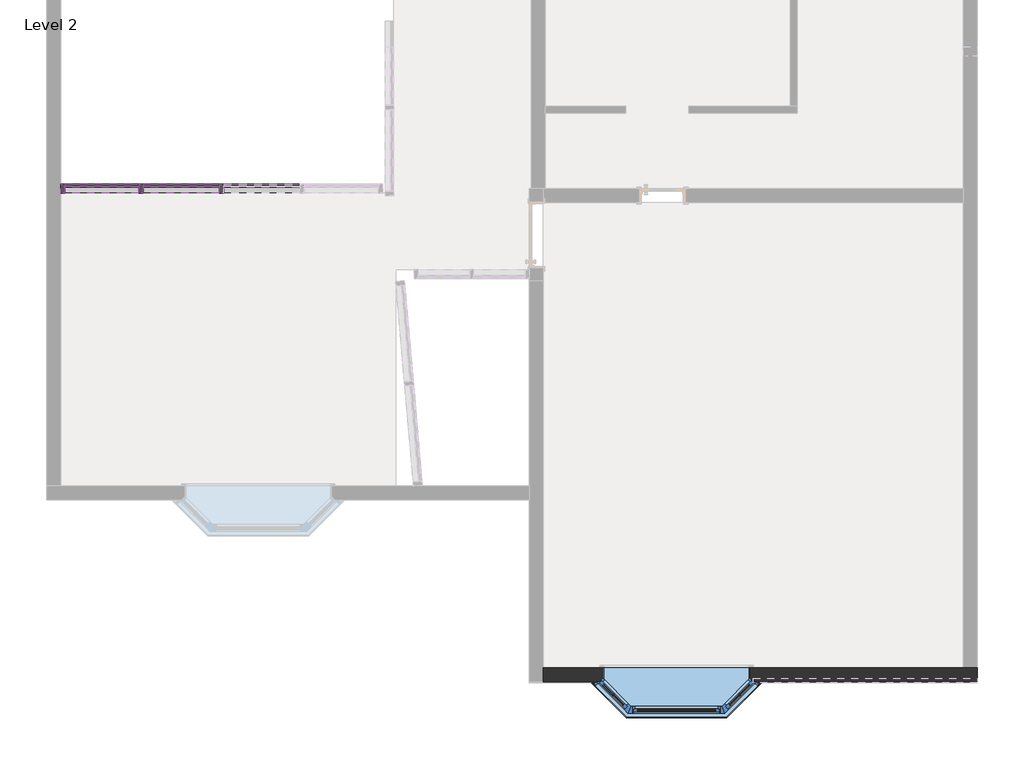
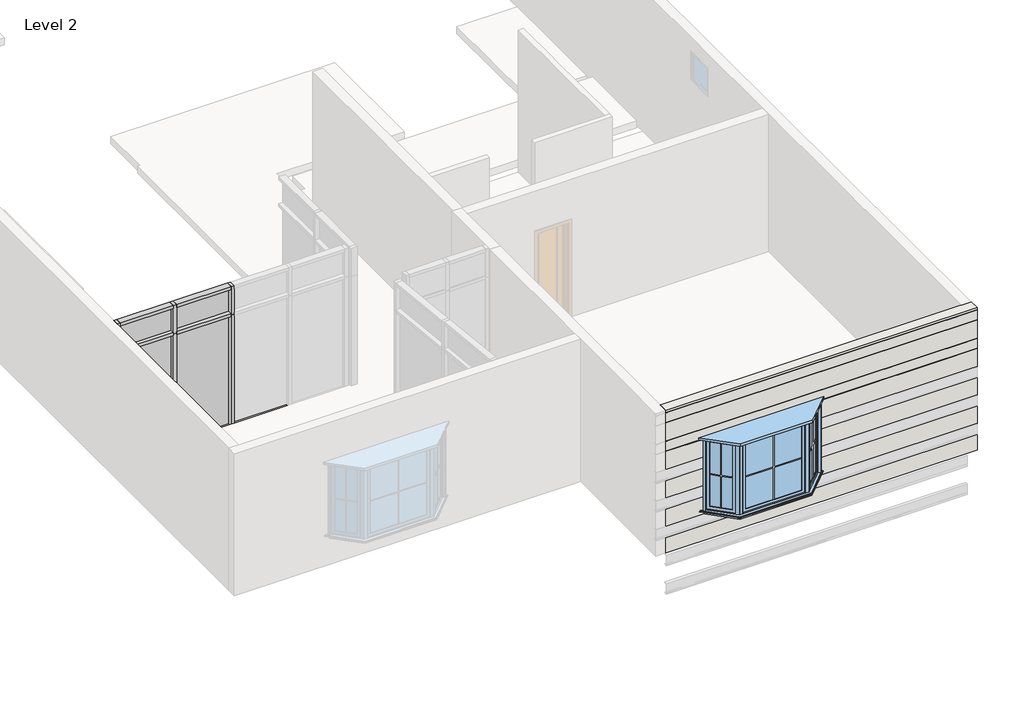
# One storey, part 1 of 5: 13 members, 4 plates, 1 wall, 1 window.
"""IFC4 building model written with IfcOpenShell, lengths in millimetres."""

from ifc_helpers import new_model, si_unit, frame, origin, place, context, project, spatial, polyline, circle_curve, ellipse_curve, transform, mapped, element, save
from ifc_brep_helpers import plane_surface, cylinder_surface, revolved_surface, advanced_brep
from components import member_47bfaf8a, member_ee409385, member_0d004d8a, member_f5e9651f, member_be44f791, member_766f1680, member_f0fea5a5, member_6e77e263, system_panel_glazed_2e981f09, system_panel_glazed_87980334, system_panel_glazed_ed20128f, system_panel_glazed_d57d3c71, window_9f89e8e4

model = new_model("IFC4")

# Units and contexts
model_context = context("Model", 3, world=origin())
ifc_project = project(units=[si_unit("LENGTHUNIT", "METRE", prefix="MILLI")], contexts=[model_context])

# Site, building, storey
site = spatial("IfcSite", under=ifc_project)
building = spatial("IfcBuilding", under=site)
storey = spatial("IfcBuildingStorey", under=building, Name="Level 2", Elevation=3048.0)

# Members
placement = place(None, origin())
member_shape = member_47bfaf8a(model_context)
element("IfcMember", 1, ObjectType="Rectangular Mullion : 2.5\" x 5\" rectangular", at=placement, inside=storey, context=model_context, shape_type="MappedRepresentation", body=[
    mapped(member_shape, transform((-50556.1380314, -2838.2913973, 6096.0), x_axis=(-1.0, 0.0, 0.0), y_axis=(0.0, -1.0, 0.0), z_axis=(0.0, 0.0, 1.0))),
])
member_2_shape = member_ee409385(model_context)
element("IfcMember", 2, ObjectType="Rectangular Mullion : 2.5\" x 5\" rectangular", at=placement, inside=storey, context=model_context, shape_type="MappedRepresentation", body=[
    mapped(member_2_shape, transform((-50556.1380314, -2838.2913973, 5486.4), x_axis=(-1.0, 0.0, 0.0), y_axis=(0.0, -1.0, 0.0), z_axis=(0.0, 0.0, 1.0))),
])
member_3_shape = member_0d004d8a(model_context)
element("IfcMember", 3, ObjectType="Rectangular Mullion : 2.5\" x 5\" rectangular", at=placement, inside=storey, context=model_context, shape_type="MappedRepresentation", body=[
    mapped(member_3_shape, transform((-49419.4880313, -2838.2913973, 6096.0), x_axis=(0.0, 0.0, 1.0), y_axis=(0.0, -1.0, 0.0), z_axis=(1.0, 0.0, 0.0))),
])
element("IfcMember", 4, ObjectType="Rectangular Mullion : 2.5\" x 5\" rectangular", at=placement, inside=storey, context=model_context, shape_type="MappedRepresentation", body=[
    mapped(member_3_shape, transform((-50492.6380314, -2838.2913973, 3048.0), x_axis=(0.0, 0.0, -1.0), y_axis=(0.0, -1.0, 0.0), z_axis=(-1.0, 0.0, 0.0))),
])
member_4_shape = member_f5e9651f(model_context)
element("IfcMember", 5, ObjectType="Rectangular Mullion : 2.5\" x 5\" rectangular", at=placement, inside=storey, context=model_context, shape_type="MappedRepresentation", body=[
    mapped(member_4_shape, transform((-48251.0880314, -2838.2913973, 6096.0), x_axis=(0.0, 0.0, 1.0), y_axis=(0.0, -1.0, 0.0), z_axis=(1.0, 0.0, 0.0))),
])
element("IfcMember", 6, ObjectType="Rectangular Mullion : 2.5\" x 5\" rectangular", at=placement, inside=storey, context=model_context, shape_type="MappedRepresentation", body=[
    mapped(member_4_shape, transform((-49355.9880313, -2838.2913973, 3048.0), x_axis=(0.0, 0.0, -1.0), y_axis=(0.0, -1.0, 0.0), z_axis=(-1.0, 0.0, 0.0))),
])
element("IfcMember", 7, ObjectType="Rectangular Mullion : 2.5\" x 5\" rectangular", at=placement, inside=storey, context=model_context, shape_type="MappedRepresentation", body=[
    mapped(member_4_shape, transform((-48187.5880314, -2838.2913973, 3048.0), x_axis=(0.0, 0.0, -1.0), y_axis=(0.0, -1.0, 0.0), z_axis=(-1.0, 0.0, 0.0))),
])
member_5_shape = member_be44f791(model_context)
element("IfcMember", 8, ObjectType="Rectangular Mullion : 2.5\" x 5\" rectangular", at=placement, inside=storey, context=model_context, shape_type="MappedRepresentation", body=[
    mapped(member_5_shape, transform((-49419.4880313, -2838.2913973, 5486.4), x_axis=(0.0, 0.0, 1.0), y_axis=(0.0, -1.0, 0.0), z_axis=(1.0, 0.0, 0.0))),
])
member_6_shape = member_766f1680(model_context)
element("IfcMember", 9, ObjectType="Rectangular Mullion : 2.5\" x 5\" rectangular", at=placement, inside=storey, context=model_context, shape_type="MappedRepresentation", body=[
    mapped(member_6_shape, transform((-48251.0880314, -2838.2913973, 5486.4), x_axis=(0.0, 0.0, 1.0), y_axis=(0.0, -1.0, 0.0), z_axis=(1.0, 0.0, 0.0))),
])
member_7_shape = member_f0fea5a5(model_context)
element("IfcMember", 10, ObjectType="Rectangular Mullion : 2.5\" x 5\" rectangular", at=placement, inside=storey, context=model_context, shape_type="MappedRepresentation", body=[
    mapped(member_7_shape, transform((-49387.7380313, -2838.2913973, 3048.0), x_axis=(1.0, 0.0, 0.0), y_axis=(0.0, -1.0, 0.0), z_axis=(0.0, 0.0, -1.0))),
])
element("IfcMember", 11, ObjectType="Rectangular Mullion : 2.5\" x 5\" rectangular", at=placement, inside=storey, context=model_context, shape_type="MappedRepresentation", body=[
    mapped(member_7_shape, transform((-48219.3380314, -2838.2913973, 3048.0), x_axis=(1.0, 0.0, 0.0), y_axis=(0.0, -1.0, 0.0), z_axis=(0.0, 0.0, -1.0))),
])
member_8_shape = member_6e77e263(model_context)
element("IfcMember", 12, ObjectType="Rectangular Mullion : 2.5\" x 5\" rectangular", at=placement, inside=storey, context=model_context, shape_type="MappedRepresentation", body=[
    mapped(member_8_shape, transform((-49387.7380313, -2838.2913973, 5486.4), x_axis=(1.0, 0.0, 0.0), y_axis=(0.0, -1.0, 0.0), z_axis=(0.0, 0.0, -1.0))),
])
element("IfcMember", 13, ObjectType="Rectangular Mullion : 2.5\" x 5\" rectangular", at=placement, inside=storey, context=model_context, shape_type="MappedRepresentation", body=[
    mapped(member_8_shape, transform((-48219.3380314, -2838.2913973, 5486.4), x_axis=(1.0, 0.0, 0.0), y_axis=(0.0, -1.0, 0.0), z_axis=(0.0, 0.0, -1.0))),
])

# Plates
system_panel_glazed_shape = system_panel_glazed_2e981f09(model_context)
element("IfcPlate", 14, ObjectType="System Panel : Glazed", at=placement, inside=storey, context=model_context, shape_type="MappedRepresentation", body=[
    mapped(system_panel_glazed_shape, transform((-49956.0630313, -2838.2913973, 3111.5), x_axis=(1.0, 0.0, 0.0), y_axis=(0.0, 1.0, 0.0), z_axis=(0.0, 0.0, 1.0))),
])
system_panel_glazed_2_shape = system_panel_glazed_87980334(model_context)
element("IfcPlate", 15, ObjectType="System Panel : Glazed", at=placement, inside=storey, context=model_context, shape_type="MappedRepresentation", body=[
    mapped(system_panel_glazed_2_shape, transform((-48803.5380313, -2838.2913973, 3111.5), x_axis=(1.0, 0.0, 0.0), y_axis=(0.0, 1.0, 0.0), z_axis=(0.0, 0.0, 1.0))),
])
system_panel_glazed_3_shape = system_panel_glazed_ed20128f(model_context)
element("IfcPlate", 16, ObjectType="System Panel : Glazed", at=placement, inside=storey, context=model_context, shape_type="MappedRepresentation", body=[
    mapped(system_panel_glazed_3_shape, transform((-49956.0630313, -2838.2913973, 5518.15), x_axis=(1.0, 0.0, 0.0), y_axis=(0.0, 1.0, 0.0), z_axis=(0.0, 0.0, 1.0))),
])
system_panel_glazed_4_shape = system_panel_glazed_d57d3c71(model_context)
element("IfcPlate", 17, ObjectType="System Panel : Glazed", at=placement, inside=storey, context=model_context, shape_type="MappedRepresentation", body=[
    mapped(system_panel_glazed_4_shape, transform((-48803.5380313, -2838.2913973, 5518.15), x_axis=(1.0, 0.0, 0.0), y_axis=(0.0, 1.0, 0.0), z_axis=(0.0, 0.0, 1.0))),
])

# Wall
element("IfcWall", 18, ObjectType="OUTER WALL 8\"", at=placement, inside=storey, context=model_context, shape_type="AdvancedBrep", body=[
    advanced_brep(
    [(-43545.7380314, -10001.0913973, 3048.0), (-37246.5380314, -10001.0913973, 3048.0), (-37246.5380314, -10001.0913973, 3390.9), (-43545.7380314, -10001.0913973, 3390.9), (-37246.5380314, -10001.0913973, 6096.0), (-43545.7380314, -10001.0913973, 6096.0), (-43545.7380314, -10001.0913973, 6057.9), (-37246.5380314, -10001.0913973, 6057.9), (-40499.1466227, -10001.0913973, 3657.6), (-42731.5294401, -10001.0913973, 3657.6), (-42731.5294401, -10001.0913973, 4000.5), (-43545.7380314, -10001.0913973, 4000.5), (-43545.7380314, -10001.0913973, 3619.5), (-37246.5380314, -10001.0913973, 3619.5), (-37246.5380314, -10001.0913973, 4000.5), (-40499.1466227, -10001.0913973, 4000.5), (-37246.5380314, -10001.0913973, 3404.84689), (-37246.5380314, -10001.0913973, 3605.55311), (-43545.7380314, -10001.0913973, 3605.55311), (-43545.7380314, -10001.0913973, 3404.84689), (-37246.5380314, -10001.0913973, 4014.44689), (-37246.5380314, -10001.0913973, 4215.15311), (-40499.1466227, -10001.0913973, 4215.15311), (-40499.1466227, -10001.0913973, 4014.44689), (-40499.1466227, -10001.0913973, 4229.1), (-37246.5380314, -10001.0913973, 4229.1), (-37246.5380314, -10001.0913973, 4610.1), (-40499.1466227, -10001.0913973, 4610.1), (-43545.7380314, -10001.0913973, 4229.1), (-42731.5294401, -10001.0913973, 4229.1), (-42731.5294401, -10001.0913973, 4610.1), (-43545.7380314, -10001.0913973, 4610.1), (-43545.7380314, -10001.0913973, 4215.15311), (-43545.7380314, -10001.0913973, 4014.44689), (-42731.5294401, -10001.0913973, 4014.44689), (-42731.5294401, -10001.0913973, 4215.15311), (-37246.5380314, -10001.0913973, 5829.3), (-43545.7380314, -10001.0913973, 5829.3), (-43545.7380314, -10001.0913973, 5448.3), (-37246.5380314, -10001.0913973, 5448.3), (-43545.7380314, -10001.0913973, 6043.95311), (-43545.7380314, -10001.0913973, 5843.24689), (-37246.5380314, -10001.0913973, 5843.24689), (-37246.5380314, -10001.0913973, 6043.95311), (-37246.5380314, -10001.0913973, 5233.64689), (-37246.5380314, -10001.0913973, 5434.35311), (-43545.7380314, -10001.0913973, 5434.35311), (-43545.7380314, -10001.0913973, 5233.64689), (-37246.5380314, -10001.0913973, 5219.7), (-40499.1466227, -10001.0913973, 5219.7), (-40499.1466227, -10001.0913973, 4838.7), (-37246.5380314, -10001.0913973, 4838.7), (-42731.5294401, -10001.0913973, 5219.7), (-43545.7380314, -10001.0913973, 5219.7), (-43545.7380314, -10001.0913973, 4838.7), (-42731.5294401, -10001.0913973, 4838.7), (-37246.5380314, -10001.0913973, 4624.04689), (-37246.5380314, -10001.0913973, 4824.75311), (-40499.1466227, -10001.0913973, 4824.75311), (-40499.1466227, -10001.0913973, 4624.04689), (-42731.5294401, -10001.0913973, 4624.04689), (-42731.5294401, -10001.0913973, 4824.75311), (-43545.7380314, -10001.0913973, 4824.75311), (-43545.7380314, -10001.0913973, 4624.04689), (-37246.5380314, -9797.8913973, 3048.0), (-37449.7380314, -9797.8913973, 3048.0), (-43545.7380314, -9797.8913973, 3048.0), (-43545.7380314, -9797.8913973, 6096.0), (-37449.7380314, -9797.8913973, 6096.0), (-37246.5380314, -9797.8913973, 6096.0), (-40548.5380314, -9797.8913973, 5232.4), (-42682.1380314, -9797.8913973, 5232.4), (-42682.1380314, -9797.8913973, 3657.6), (-40548.5380314, -9797.8913973, 3657.6), (-43545.7380314, -9952.7297973, 3390.9), (-43545.7380314, -9952.7297973, 3392.2796758), (-43545.7380314, -9957.1126065, 3397.4534103), (-43545.7380314, -9999.9711789, 3404.59652), (-43545.7380314, -9999.9711789, 3605.80348), (-43545.7380314, -9957.1126065, 3612.9465897), (-43545.7380314, -9952.7297973, 3618.1203242), (-43545.7380314, -9952.7297973, 3619.5), (-43545.7380314, -9952.7297973, 4000.5), (-43545.7380314, -9952.7297973, 4001.8796758), (-43545.7380314, -9957.1126065, 4007.0534103), (-43545.7380314, -9999.9711789, 4014.19652), (-43545.7380314, -9999.9711789, 4215.40348), (-43545.7380314, -9957.1126065, 4222.5465897), (-43545.7380314, -9952.7297973, 4227.7203242), (-43545.7380314, -9952.7297973, 4229.1), (-43545.7380314, -9952.7297973, 4610.1), (-43545.7380314, -9952.7297973, 4611.4796758), (-43545.7380314, -9957.1126065, 4616.6534103), (-43545.7380314, -9999.9711789, 4623.79652), (-43545.7380314, -9999.9711789, 4825.00348), (-43545.7380314, -9957.1126065, 4832.1465897), (-43545.7380314, -9952.7297973, 4837.3203242), (-43545.7380314, -9952.7297973, 4838.7), (-43545.7380314, -9952.7297973, 5219.7), (-43545.7380314, -9952.7297973, 5221.0796758), (-43545.7380314, -9957.1126065, 5226.2534103), (-43545.7380314, -9999.9711789, 5233.39652), (-43545.7380314, -9999.9711789, 5434.60348), (-43545.7380314, -9957.1126065, 5441.7465897), (-43545.7380314, -9952.7297973, 5446.9203242), (-43545.7380314, -9952.7297973, 5448.3), (-43545.7380314, -9952.7297973, 5829.3), (-43545.7380314, -9952.7297973, 5830.6796758), (-43545.7380314, -9957.1126065, 5835.8534103), (-43545.7380314, -9999.9711789, 5842.99652), (-43545.7380314, -9999.9711789, 6044.20348), (-43545.7380314, -9957.1126065, 6051.3465897), (-43545.7380314, -9952.7297973, 6056.5203242), (-43545.7380314, -9952.7297973, 6057.9), (-37246.5380314, -9952.7297973, 6057.9), (-37246.5380314, -9952.7297973, 6056.5203242), (-37246.5380314, -9957.1126065, 6051.3465897), (-37246.5380314, -9999.9711789, 6044.20348), (-37246.5380314, -9999.9711789, 5842.99652), (-37246.5380314, -9957.1126065, 5835.8534103), (-37246.5380314, -9952.7297973, 5830.6796758), (-37246.5380314, -9952.7297973, 5829.3), (-37246.5380314, -9952.7297973, 5448.3), (-37246.5380314, -9952.7297973, 5446.9203242), (-37246.5380314, -9957.1126065, 5441.7465897), (-37246.5380314, -9999.9711789, 5434.60348), (-37246.5380314, -9999.9711789, 5233.39652), (-37246.5380314, -9957.1126065, 5226.2534103), (-37246.5380314, -9952.7297973, 5221.0796758), (-37246.5380314, -9952.7297973, 5219.7), (-37246.5380314, -9952.7297973, 4838.7), (-37246.5380314, -9952.7297973, 4837.3203242), (-37246.5380314, -9957.1126065, 4832.1465897), (-37246.5380314, -9999.9711789, 4825.00348), (-37246.5380314, -9999.9711789, 4623.79652), (-37246.5380314, -9957.1126065, 4616.6534103), (-37246.5380314, -9952.7297973, 4611.4796758), (-37246.5380314, -9952.7297973, 4610.1), (-37246.5380314, -9952.7297973, 4229.1), (-37246.5380314, -9952.7297973, 4227.7203242), (-37246.5380314, -9957.1126065, 4222.5465897), (-37246.5380314, -9999.9711789, 4215.40348), (-37246.5380314, -9999.9711789, 4014.19652), (-37246.5380314, -9957.1126065, 4007.0534103), (-37246.5380314, -9952.7297973, 4001.8796758), (-37246.5380314, -9952.7297973, 4000.5), (-37246.5380314, -9952.7297973, 3619.5), (-37246.5380314, -9952.7297973, 3618.1203242), (-37246.5380314, -9957.1126065, 3612.9465897), (-37246.5380314, -9999.9711789, 3605.80348), (-37246.5380314, -9999.9711789, 3404.59652), (-37246.5380314, -9957.1126065, 3397.4534103), (-37246.5380314, -9952.7297973, 3392.2796758), (-37246.5380314, -9952.7297973, 3390.9), (-42682.1380314, -9951.6999886, 5232.4), (-40548.5380314, -9951.6999886, 5232.4), (-40506.2459493, -9993.9920707, 5232.4), (-42724.4301136, -9993.9920707, 5232.4), (-40548.5380314, -9951.6999886, 3657.6), (-42682.1380314, -9951.6999886, 3657.6), (-42687.5506493, -9957.1126065, 5226.2534103), (-42683.1678401, -9952.7297973, 5221.0796758), (-42683.1678401, -9952.7297973, 5219.7), (-40547.5082227, -9952.7297973, 5219.7), (-40547.5082227, -9952.7297973, 5221.0796758), (-40543.1254136, -9957.1126065, 5226.2534103), (-40499.1466227, -9952.7297973, 4227.7203242), (-40499.1466227, -9952.7297973, 4229.1), (-40499.1466227, -9999.9711789, 4215.40348), (-40499.1466227, -9957.1126065, 4222.5465897), (-40499.1466227, -9957.1126065, 4007.0534103), (-40499.1466227, -9999.9711789, 4014.19652), (-40499.1466227, -9952.7297973, 4000.5), (-40499.1466227, -9952.7297973, 4001.8796758), (-42731.5294401, -9952.7297973, 4001.8796758), (-42731.5294401, -9952.7297973, 4000.5), (-42731.5294401, -9999.9711789, 4014.19652), (-42731.5294401, -9957.1126065, 4007.0534103), (-42731.5294401, -9957.1126065, 4222.5465897), (-42731.5294401, -9999.9711789, 4215.40348), (-42731.5294401, -9952.7297973, 4229.1), (-42731.5294401, -9952.7297973, 4227.7203242), (-40499.1466227, -9952.7297973, 4837.3203242), (-40499.1466227, -9952.7297973, 4838.7), (-40499.1466227, -9999.9711789, 4825.00348), (-40499.1466227, -9957.1126065, 4832.1465897), (-40499.1466227, -9957.1126065, 4616.6534103), (-40499.1466227, -9999.9711789, 4623.79652), (-40499.1466227, -9952.7297973, 4610.1), (-40499.1466227, -9952.7297973, 4611.4796758), (-42731.5294401, -9952.7297973, 4611.4796758), (-42731.5294401, -9952.7297973, 4610.1), (-42731.5294401, -9999.9711789, 4623.79652), (-42731.5294401, -9957.1126065, 4616.6534103), (-42731.5294401, -9957.1126065, 4832.1465897), (-42731.5294401, -9999.9711789, 4825.00348), (-42731.5294401, -9952.7297973, 4838.7), (-42731.5294401, -9952.7297973, 4837.3203242)],
    [
        (0, 1),
        (1, 2),
        (2, 3),
        (3, 0),
        (4, 5),
        (5, 6),
        (6, 7),
        (7, 4),
        (8, 9),
        (9, 10),
        (10, 11),
        (11, 12),
        (12, 13),
        (13, 14),
        (14, 15),
        (15, 8),
        (16, 17),
        (17, 18),
        (18, 19),
        (19, 16),
        (20, 21),
        (21, 22),
        (22, 23),
        (23, 20),
        (24, 25),
        (25, 26),
        (26, 27),
        (27, 24),
        (28, 29),
        (29, 30),
        (30, 31),
        (31, 28),
        (32, 33),
        (33, 34),
        (34, 35),
        (35, 32),
        (36, 37),
        (37, 38),
        (38, 39),
        (39, 36),
        (40, 41),
        (41, 42),
        (42, 43),
        (43, 40),
        (44, 45),
        (45, 46),
        (46, 47),
        (47, 44),
        (48, 49),
        (49, 50),
        (50, 51),
        (51, 48),
        (52, 53),
        (53, 54),
        (54, 55),
        (55, 52),
        (56, 57),
        (57, 58),
        (58, 59),
        (59, 56),
        (60, 61),
        (61, 62),
        (62, 63),
        (63, 60),
        (64, 65),
        (65, 66),
        (66, 67),
        (67, 68),
        (68, 69),
        (69, 64),
        (70, 71),
        (71, 72),
        (72, 73),
        (73, 70),
        (0, 66),
        (64, 1),
        (4, 69),
        (67, 5),
        (3, 74),
        (74, 75),
        (75, 76, circle_curve(frame((-43545.7380314, -9957.9748973, 3392.2796758), z_axis=(1.0, 0.0, 0.0), x_axis=(0.0, 1.0, 0.0)), 5.2451)),
        (76, 77),
        (77, 19, circle_curve(frame((-43545.7380314, -9998.2465973, 3414.943989), z_axis=(-1.0, 0.0, 0.0), x_axis=(0.0, 1.0, 0.0)), 10.4902)),
        (18, 78, circle_curve(frame((-43545.7380314, -9998.2465973, 3595.456011), z_axis=(-1.0, 0.0, 0.0), x_axis=(0.0, 1.0, 0.0)), 10.4902)),
        (78, 79),
        (79, 80, circle_curve(frame((-43545.7380314, -9957.9748973, 3618.1203242), z_axis=(1.0, 0.0, 0.0), x_axis=(0.0, 1.0, 0.0)), 5.2451)),
        (80, 81),
        (81, 12),
        (11, 82),
        (82, 83),
        (83, 84, circle_curve(frame((-43545.7380314, -9957.9748973, 4001.8796758), z_axis=(1.0, 0.0, 0.0), x_axis=(0.0, 1.0, 0.0)), 5.2451)),
        (84, 85),
        (85, 33, circle_curve(frame((-43545.7380314, -9998.2465973, 4024.543989), z_axis=(-1.0, 0.0, 0.0), x_axis=(0.0, 1.0, 0.0)), 10.4902)),
        (32, 86, circle_curve(frame((-43545.7380314, -9998.2465973, 4205.056011), z_axis=(-1.0, 0.0, 0.0), x_axis=(0.0, 1.0, 0.0)), 10.4902)),
        (86, 87),
        (87, 88, circle_curve(frame((-43545.7380314, -9957.9748973, 4227.7203242), z_axis=(1.0, 0.0, 0.0), x_axis=(0.0, 1.0, 0.0)), 5.2451)),
        (88, 89),
        (89, 28),
        (31, 90),
        (90, 91),
        (91, 92, circle_curve(frame((-43545.7380314, -9957.9748973, 4611.4796758), z_axis=(1.0, 0.0, 0.0), x_axis=(0.0, 1.0, 0.0)), 5.2451)),
        (92, 93),
        (93, 63, circle_curve(frame((-43545.7380314, -9998.2465973, 4634.143989), z_axis=(-1.0, 0.0, 0.0), x_axis=(0.0, 1.0, 0.0)), 10.4902)),
        (62, 94, circle_curve(frame((-43545.7380314, -9998.2465973, 4814.656011), z_axis=(-1.0, 0.0, 0.0), x_axis=(0.0, 1.0, 0.0)), 10.4902)),
        (94, 95),
        (95, 96, circle_curve(frame((-43545.7380314, -9957.9748973, 4837.3203242), z_axis=(1.0, 0.0, 0.0), x_axis=(0.0, 1.0, 0.0)), 5.2451)),
        (96, 97),
        (97, 54),
        (53, 98),
        (98, 99),
        (99, 100, circle_curve(frame((-43545.7380314, -9957.9748973, 5221.0796758), z_axis=(1.0, 0.0, 0.0), x_axis=(0.0, 1.0, 0.0)), 5.2451)),
        (100, 101),
        (101, 47, circle_curve(frame((-43545.7380314, -9998.2465973, 5243.743989), z_axis=(-1.0, 0.0, 0.0), x_axis=(0.0, 1.0, 0.0)), 10.4902)),
        (46, 102, circle_curve(frame((-43545.7380314, -9998.2465973, 5424.256011), z_axis=(-1.0, 0.0, 0.0), x_axis=(0.0, 1.0, 0.0)), 10.4902)),
        (102, 103),
        (103, 104, circle_curve(frame((-43545.7380314, -9957.9748973, 5446.9203242), z_axis=(1.0, 0.0, 0.0), x_axis=(0.0, 1.0, 0.0)), 5.2451)),
        (104, 105),
        (105, 38),
        (37, 106),
        (106, 107),
        (107, 108, circle_curve(frame((-43545.7380314, -9957.9748973, 5830.6796758), z_axis=(1.0, 0.0, 0.0), x_axis=(0.0, 1.0, 0.0)), 5.2451)),
        (108, 109),
        (109, 41, circle_curve(frame((-43545.7380314, -9998.2465973, 5853.343989), z_axis=(-1.0, 0.0, 0.0), x_axis=(0.0, 1.0, 0.0)), 10.4902)),
        (40, 110, circle_curve(frame((-43545.7380314, -9998.2465973, 6033.856011), z_axis=(-1.0, 0.0, 0.0), x_axis=(0.0, 1.0, 0.0)), 10.4902)),
        (110, 111),
        (111, 112, circle_curve(frame((-43545.7380314, -9957.9748973, 6056.5203242), z_axis=(1.0, 0.0, 0.0), x_axis=(0.0, 1.0, 0.0)), 5.2451)),
        (112, 113),
        (113, 6),
        (7, 114),
        (114, 115),
        (115, 116, circle_curve(frame((-37246.5380314, -9957.9748973, 6056.5203242), z_axis=(-1.0, 0.0, 0.0), x_axis=(0.0, 1.0, 0.0)), 5.2451)),
        (116, 117),
        (117, 43, circle_curve(frame((-37246.5380314, -9998.2465973, 6033.856011), z_axis=(1.0, 0.0, 0.0), x_axis=(0.0, 1.0, 0.0)), 10.4902)),
        (42, 118, circle_curve(frame((-37246.5380314, -9998.2465973, 5853.343989), z_axis=(1.0, 0.0, 0.0), x_axis=(0.0, 1.0, 0.0)), 10.4902)),
        (118, 119),
        (119, 120, circle_curve(frame((-37246.5380314, -9957.9748973, 5830.6796758), z_axis=(-1.0, 0.0, 0.0), x_axis=(0.0, 1.0, 0.0)), 5.2451)),
        (120, 121),
        (121, 36),
        (39, 122),
        (122, 123),
        (123, 124, circle_curve(frame((-37246.5380314, -9957.9748973, 5446.9203242), z_axis=(-1.0, 0.0, 0.0), x_axis=(0.0, 1.0, 0.0)), 5.2451)),
        (124, 125),
        (125, 45, circle_curve(frame((-37246.5380314, -9998.2465973, 5424.256011), z_axis=(1.0, 0.0, 0.0), x_axis=(0.0, 1.0, 0.0)), 10.4902)),
        (44, 126, circle_curve(frame((-37246.5380314, -9998.2465973, 5243.743989), z_axis=(1.0, 0.0, 0.0), x_axis=(0.0, 1.0, 0.0)), 10.4902)),
        (126, 127),
        (127, 128, circle_curve(frame((-37246.5380314, -9957.9748973, 5221.0796758), z_axis=(-1.0, 0.0, 0.0), x_axis=(0.0, 1.0, 0.0)), 5.2451)),
        (128, 129),
        (129, 48),
        (51, 130),
        (130, 131),
        (131, 132, circle_curve(frame((-37246.5380314, -9957.9748973, 4837.3203242), z_axis=(-1.0, 0.0, 0.0), x_axis=(0.0, 1.0, 0.0)), 5.2451)),
        (132, 133),
        (133, 57, circle_curve(frame((-37246.5380314, -9998.2465973, 4814.656011), z_axis=(1.0, 0.0, 0.0), x_axis=(0.0, 1.0, 0.0)), 10.4902)),
        (56, 134, circle_curve(frame((-37246.5380314, -9998.2465973, 4634.143989), z_axis=(1.0, 0.0, 0.0), x_axis=(0.0, 1.0, 0.0)), 10.4902)),
        (134, 135),
        (135, 136, circle_curve(frame((-37246.5380314, -9957.9748973, 4611.4796758), z_axis=(-1.0, 0.0, 0.0), x_axis=(0.0, 1.0, 0.0)), 5.2451)),
        (136, 137),
        (137, 26),
        (25, 138),
        (138, 139),
        (139, 140, circle_curve(frame((-37246.5380314, -9957.9748973, 4227.7203242), z_axis=(-1.0, 0.0, 0.0), x_axis=(0.0, 1.0, 0.0)), 5.2451)),
        (140, 141),
        (141, 21, circle_curve(frame((-37246.5380314, -9998.2465973, 4205.056011), z_axis=(1.0, 0.0, 0.0), x_axis=(0.0, 1.0, 0.0)), 10.4902)),
        (20, 142, circle_curve(frame((-37246.5380314, -9998.2465973, 4024.543989), z_axis=(1.0, 0.0, 0.0), x_axis=(0.0, 1.0, 0.0)), 10.4902)),
        (142, 143),
        (143, 144, circle_curve(frame((-37246.5380314, -9957.9748973, 4001.8796758), z_axis=(-1.0, 0.0, 0.0), x_axis=(0.0, 1.0, 0.0)), 5.2451)),
        (144, 145),
        (145, 14),
        (13, 146),
        (146, 147),
        (147, 148, circle_curve(frame((-37246.5380314, -9957.9748973, 3618.1203242), z_axis=(-1.0, 0.0, 0.0), x_axis=(0.0, 1.0, 0.0)), 5.2451)),
        (148, 149),
        (149, 17, circle_curve(frame((-37246.5380314, -9998.2465973, 3595.456011), z_axis=(1.0, 0.0, 0.0), x_axis=(0.0, 1.0, 0.0)), 10.4902)),
        (16, 150, circle_curve(frame((-37246.5380314, -9998.2465973, 3414.943989), z_axis=(1.0, 0.0, 0.0), x_axis=(0.0, 1.0, 0.0)), 10.4902)),
        (150, 151),
        (151, 152, circle_curve(frame((-37246.5380314, -9957.9748973, 3392.2796758), z_axis=(-1.0, 0.0, 0.0), x_axis=(0.0, 1.0, 0.0)), 5.2451)),
        (152, 153),
        (153, 2),
        (154, 71),
        (70, 155),
        (155, 156),
        (156, 157),
        (157, 154),
        (158, 73),
        (72, 159),
        (159, 9),
        (8, 158),
        (158, 155),
        (154, 159),
        (157, 160),
        (160, 161, ellipse_curve(frame((-42688.4129401, -9957.9748973, 5221.0796758), z_axis=(-0.7071067811865455, 0.7071067811865496, 0.0), x_axis=(-0.7071067811865497, -0.7071067811865455, 0.0)), 7.4176916, 5.2451)),
        (161, 162),
        (162, 52),
        (55, 61),
        (60, 30),
        (29, 35),
        (34, 10),
        (15, 23),
        (22, 24),
        (27, 59),
        (58, 50),
        (49, 163),
        (163, 164),
        (164, 165, ellipse_curve(frame((-40542.2631227, -9957.9748973, 5221.0796758), z_axis=(0.7071067811865509, 0.7071067811865442, 0.0), x_axis=(-0.707106781186544, 0.707106781186551, 0.0)), 7.4176916, 5.2451)),
        (165, 156),
        (81, 146),
        (80, 147),
        (79, 148),
        (78, 149),
        (77, 150),
        (76, 151),
        (75, 152),
        (74, 153),
        (166, 167),
        (167, 24),
        (22, 168, circle_curve(frame((-40499.1466227, -9998.2465973, 4205.056011), z_axis=(-1.0, 0.0, 0.0), x_axis=(0.0, 1.0, 0.0)), 10.4902)),
        (168, 169),
        (169, 166, circle_curve(frame((-40499.1466227, -9957.9748973, 4227.7203242), z_axis=(1.0, 0.0, 0.0), x_axis=(0.0, 1.0, 0.0)), 5.2451)),
        (170, 171),
        (171, 23, circle_curve(frame((-40499.1466227, -9998.2465973, 4024.543989), z_axis=(-1.0, 0.0, 0.0), x_axis=(0.0, 1.0, 0.0)), 10.4902)),
        (15, 172),
        (172, 173),
        (173, 170, circle_curve(frame((-40499.1466227, -9957.9748973, 4001.8796758), z_axis=(1.0, 0.0, 0.0), x_axis=(0.0, 1.0, 0.0)), 5.2451)),
        (167, 138),
        (166, 139),
        (169, 140),
        (168, 141),
        (171, 142),
        (170, 143),
        (173, 144),
        (172, 145),
        (174, 175),
        (175, 10),
        (34, 176, circle_curve(frame((-42731.5294401, -9998.2465973, 4024.543989), z_axis=(1.0, 0.0, 0.0), x_axis=(0.0, 1.0, 0.0)), 10.4902)),
        (176, 177),
        (177, 174, circle_curve(frame((-42731.5294401, -9957.9748973, 4001.8796758), z_axis=(-1.0, 0.0, 0.0), x_axis=(0.0, 1.0, 0.0)), 5.2451)),
        (178, 179),
        (179, 35, circle_curve(frame((-42731.5294401, -9998.2465973, 4205.056011), z_axis=(1.0, 0.0, 0.0), x_axis=(0.0, 1.0, 0.0)), 10.4902)),
        (29, 180),
        (180, 181),
        (181, 178, circle_curve(frame((-42731.5294401, -9957.9748973, 4227.7203242), z_axis=(-1.0, 0.0, 0.0), x_axis=(0.0, 1.0, 0.0)), 5.2451)),
        (89, 180),
        (88, 181),
        (87, 178),
        (86, 179),
        (85, 176),
        (84, 177),
        (83, 174),
        (82, 175),
        (113, 114),
        (112, 115),
        (111, 116),
        (110, 117),
        (109, 118),
        (108, 119),
        (107, 120),
        (106, 121),
        (105, 122),
        (104, 123),
        (103, 124),
        (102, 125),
        (101, 126),
        (100, 160),
        (165, 127),
        (99, 161),
        (164, 128),
        (98, 162),
        (163, 129),
        (182, 183),
        (183, 50),
        (58, 184, circle_curve(frame((-40499.1466227, -9998.2465973, 4814.656011), z_axis=(-1.0, 0.0, 0.0), x_axis=(0.0, 1.0, 0.0)), 10.4902)),
        (184, 185),
        (185, 182, circle_curve(frame((-40499.1466227, -9957.9748973, 4837.3203242), z_axis=(1.0, 0.0, 0.0), x_axis=(0.0, 1.0, 0.0)), 5.2451)),
        (186, 187),
        (187, 59, circle_curve(frame((-40499.1466227, -9998.2465973, 4634.143989), z_axis=(-1.0, 0.0, 0.0), x_axis=(0.0, 1.0, 0.0)), 10.4902)),
        (27, 188),
        (188, 189),
        (189, 186, circle_curve(frame((-40499.1466227, -9957.9748973, 4611.4796758), z_axis=(1.0, 0.0, 0.0), x_axis=(0.0, 1.0, 0.0)), 5.2451)),
        (183, 130),
        (182, 131),
        (185, 132),
        (184, 133),
        (187, 134),
        (186, 135),
        (189, 136),
        (188, 137),
        (190, 191),
        (191, 30),
        (60, 192, circle_curve(frame((-42731.5294401, -9998.2465973, 4634.143989), z_axis=(1.0, 0.0, 0.0), x_axis=(0.0, 1.0, 0.0)), 10.4902)),
        (192, 193),
        (193, 190, circle_curve(frame((-42731.5294401, -9957.9748973, 4611.4796758), z_axis=(-1.0, 0.0, 0.0), x_axis=(0.0, 1.0, 0.0)), 5.2451)),
        (194, 195),
        (195, 61, circle_curve(frame((-42731.5294401, -9998.2465973, 4814.656011), z_axis=(1.0, 0.0, 0.0), x_axis=(0.0, 1.0, 0.0)), 10.4902)),
        (55, 196),
        (196, 197),
        (197, 194, circle_curve(frame((-42731.5294401, -9957.9748973, 4837.3203242), z_axis=(-1.0, 0.0, 0.0), x_axis=(0.0, 1.0, 0.0)), 5.2451)),
        (97, 196),
        (96, 197),
        (95, 194),
        (94, 195),
        (93, 192),
        (92, 193),
        (91, 190),
        (90, 191),
    ],
    [
        plane_surface(frame((-43748.9380314, -10001.0913973, 3048.0), z_axis=(0.0, -1.0, 0.0), x_axis=(1.0, 0.0, 0.0))),
        plane_surface(frame((-43748.9380314, -9797.8913973, 3048.0), z_axis=(0.0, 1.0, 0.0), x_axis=(-1.0, 0.0, 0.0))),
        plane_surface(frame((-43647.3380314, -10001.0913973, 3048.0), z_axis=(0.0, 0.0, -1.0), x_axis=(0.0, 1.0, 0.0))),
        plane_surface(frame((-37348.1380314, -10001.0913973, 6096.0), z_axis=(0.0, 0.0, 1.0), x_axis=(0.0, 1.0, 0.0))),
        plane_surface(frame((-43545.7380314, -4081.0930974, 3048.0), z_axis=(-1.0, 0.0, 0.0), x_axis=(0.0, 1.0, 0.0))),
        plane_surface(frame((-37246.5380314, -10001.0913973, 3048.0), z_axis=(1.0, 0.0, 0.0), x_axis=(0.0, 1.0, 0.0))),
        plane_surface(frame((-40548.5380314, -9951.6999886, 5232.4), z_axis=(0.0, 0.0, -1.0), x_axis=(0.0, 1.0, 0.0))),
        plane_surface(frame((-40548.5380314, -9951.6999886, 3657.6), z_axis=(0.0, 0.0, 1.0), x_axis=(0.0, -1.0, 0.0))),
        plane_surface(frame((-40548.5380314, -9951.6999886, 5232.4), z_axis=(-1.0, 0.0, 0.0), x_axis=(0.0, 0.0, -1.0))),
        plane_surface(frame((-42682.1380314, -9797.8913973, 5232.4), z_axis=(1.0, 0.0, 0.0), x_axis=(0.0, 0.0, -1.0))),
        plane_surface(frame((-42682.1380314, -9951.6999886, 5232.4), z_axis=(0.7071067811865455, -0.7071067811865496, 0.0), x_axis=(0.0, 0.0, -1.0))),
        plane_surface(frame((-40499.1466227, -10001.0913973, 5232.4), z_axis=(-0.7071067811865509, -0.7071067811865442, 0.0), x_axis=(0.0, 0.0, -1.0))),
        plane_surface(frame((-43748.9380314, -10015.9757973, 3619.5), z_axis=(0.0, 0.0, -1.0), x_axis=(1.0, 0.0, 0.0))),
        plane_surface(frame((-43748.9380314, -9952.7297973, 3619.5), z_axis=(0.0, -1.0, 0.0), x_axis=(1.0, 0.0, 0.0))),
        revolved_surface(polyline([(-43545.7380314, -9952.7297973, 3618.1203242), (-37246.5380314, -9952.7297973, 3618.1203242)]), (-43748.9380314, -9957.9748973, 3618.1203242), (-1.0, 0.0, 0.0)),
        plane_surface(frame((-43748.9380314, -9980.7332973, 3609.0098), z_axis=(0.0, -0.16439930721687146, 0.9863938705135048), x_axis=(1.0, 0.0, 0.0))),
        cylinder_surface(frame((-43748.9380314, -9998.2465973, 3595.456011), z_axis=(1.0, 0.0, 0.0), x_axis=(0.0, 1.0, 0.0)), 10.4902),
        cylinder_surface(frame((-43748.9380314, -9998.2465973, 3414.943989), z_axis=(1.0, 0.0, 0.0), x_axis=(0.0, 1.0, 0.0)), 10.4902),
        plane_surface(frame((-43748.9380314, -9980.7332973, 3401.3902), z_axis=(0.0, -0.16439930721687793, -0.9863938705135037), x_axis=(1.0, 0.0, 0.0))),
        revolved_surface(polyline([(-43545.7380314, -9952.7297973, 3392.2796758), (-37246.5380314, -9952.7297973, 3392.2796758)]), (-43748.9380314, -9957.9748973, 3392.2796758), (-1.0, 0.0, 0.0)),
        plane_surface(frame((-43748.9380314, -9952.7297973, 3392.2796758), z_axis=(0.0, -1.0, 0.0), x_axis=(1.0, 0.0, 0.0))),
        plane_surface(frame((-43748.9380314, -9952.7297973, 3390.9), z_axis=(0.0, 0.0, 1.0), x_axis=(1.0, 0.0, 0.0))),
        plane_surface(frame((-40499.1466227, -10001.0913973, 3990.6898298), z_axis=(1.0, 0.0, 0.0), x_axis=(0.0, 1.0, 0.0))),
        plane_surface(frame((-40499.1466227, -10015.9757973, 4229.1), z_axis=(0.0, 0.0, -1.0), x_axis=(1.0, 0.0, 0.0))),
        plane_surface(frame((-40499.1466227, -9952.7297973, 4229.1), z_axis=(0.0, -1.0, 0.0), x_axis=(1.0, 0.0, 0.0))),
        revolved_surface(polyline([(-40499.1466227, -9952.7297973, 4227.7203242), (-37246.5380314, -9952.7297973, 4227.7203242)]), (-40499.1466227, -9957.9748973, 4227.7203242), (-1.0, 0.0, 0.0)),
        plane_surface(frame((-40499.1466227, -9980.7332973, 4218.6098), z_axis=(0.0, -0.16439930721687146, 0.9863938705135048), x_axis=(1.0, 0.0, 0.0))),
        cylinder_surface(frame((-40499.1466227, -9998.2465973, 4205.056011), z_axis=(1.0, 0.0, 0.0), x_axis=(0.0, 1.0, 0.0)), 10.4902),
        cylinder_surface(frame((-40499.1466227, -9998.2465973, 4024.543989), z_axis=(1.0, 0.0, 0.0), x_axis=(0.0, 1.0, 0.0)), 10.4902),
        plane_surface(frame((-40499.1466227, -9980.7332973, 4010.9902), z_axis=(0.0, -0.16439930721687793, -0.9863938705135037), x_axis=(1.0, 0.0, 0.0))),
        revolved_surface(polyline([(-40499.1466227, -9952.7297973, 4001.8796758), (-37246.5380314, -9952.7297973, 4001.8796758)]), (-40499.1466227, -9957.9748973, 4001.8796758), (-1.0, 0.0, 0.0)),
        plane_surface(frame((-40499.1466227, -9952.7297973, 4001.8796758), z_axis=(0.0, -1.0, 0.0), x_axis=(1.0, 0.0, 0.0))),
        plane_surface(frame((-40499.1466227, -9952.7297973, 4000.5), z_axis=(0.0, 0.0, 1.0), x_axis=(1.0, 0.0, 0.0))),
        plane_surface(frame((-42731.5294401, -10001.0913973, 3990.6898298), z_axis=(-1.0, 0.0, 0.0), x_axis=(0.0, 1.0, 0.0))),
        plane_surface(frame((-43748.9380314, -10015.9757973, 4229.1), z_axis=(0.0, 0.0, -1.0), x_axis=(1.0, 0.0, 0.0))),
        plane_surface(frame((-43748.9380314, -9952.7297973, 4229.1), z_axis=(0.0, -1.0, 0.0), x_axis=(1.0, 0.0, 0.0))),
        revolved_surface(polyline([(-43545.7380314, -9952.7297973, 4227.7203242), (-42731.5294401, -9952.7297973, 4227.7203242)]), (-43748.9380314, -9957.9748973, 4227.7203242), (-1.0, 0.0, 0.0)),
        plane_surface(frame((-43748.9380314, -9980.7332973, 4218.6098), z_axis=(0.0, -0.16439930721687146, 0.9863938705135048), x_axis=(1.0, 0.0, 0.0))),
        cylinder_surface(frame((-43748.9380314, -9998.2465973, 4205.056011), z_axis=(1.0, 0.0, 0.0), x_axis=(0.0, 1.0, 0.0)), 10.4902),
        cylinder_surface(frame((-43748.9380314, -9998.2465973, 4024.543989), z_axis=(1.0, 0.0, 0.0), x_axis=(0.0, 1.0, 0.0)), 10.4902),
        plane_surface(frame((-43748.9380314, -9980.7332973, 4010.9902), z_axis=(0.0, -0.16439930721687793, -0.9863938705135037), x_axis=(1.0, 0.0, 0.0))),
        revolved_surface(polyline([(-43545.7380314, -9952.7297973, 4001.8796758), (-42731.5294401, -9952.7297973, 4001.8796758)]), (-43748.9380314, -9957.9748973, 4001.8796758), (-1.0, 0.0, 0.0)),
        plane_surface(frame((-43748.9380314, -9952.7297973, 4001.8796758), z_axis=(0.0, -1.0, 0.0), x_axis=(1.0, 0.0, 0.0))),
        plane_surface(frame((-43748.9380314, -9952.7297973, 4000.5), z_axis=(0.0, 0.0, 1.0), x_axis=(1.0, 0.0, 0.0))),
        plane_surface(frame((-43748.9380314, -10015.9757973, 6057.9), z_axis=(0.0, 0.0, -1.0), x_axis=(1.0, 0.0, 0.0))),
        plane_surface(frame((-43748.9380314, -9952.7297973, 6057.9), z_axis=(0.0, -1.0, 0.0), x_axis=(1.0, 0.0, 0.0))),
        revolved_surface(polyline([(-43545.7380314, -9952.7297973, 6056.5203242), (-37246.5380314, -9952.7297973, 6056.5203242)]), (-43748.9380314, -9957.9748973, 6056.5203242), (-1.0, 0.0, 0.0)),
        plane_surface(frame((-43748.9380314, -9980.7332973, 6047.4098), z_axis=(0.0, -0.16439930721687146, 0.9863938705135048), x_axis=(1.0, 0.0, 0.0))),
        cylinder_surface(frame((-43748.9380314, -9998.2465973, 6033.856011), z_axis=(1.0, 0.0, 0.0), x_axis=(0.0, 1.0, 0.0)), 10.4902),
        cylinder_surface(frame((-43748.9380314, -9998.2465973, 5853.343989), z_axis=(1.0, 0.0, 0.0), x_axis=(0.0, 1.0, 0.0)), 10.4902),
        plane_surface(frame((-43748.9380314, -9980.7332973, 5839.7902), z_axis=(0.0, -0.16439930721687793, -0.9863938705135037), x_axis=(1.0, 0.0, 0.0))),
        revolved_surface(polyline([(-43545.7380314, -9952.7297973, 5830.6796758), (-37246.5380314, -9952.7297973, 5830.6796758)]), (-43748.9380314, -9957.9748973, 5830.6796758), (-1.0, 0.0, 0.0)),
        plane_surface(frame((-43748.9380314, -9952.7297973, 5830.6796758), z_axis=(0.0, -1.0, 0.0), x_axis=(1.0, 0.0, 0.0))),
        plane_surface(frame((-43748.9380314, -9952.7297973, 5829.3), z_axis=(0.0, 0.0, 1.0), x_axis=(1.0, 0.0, 0.0))),
        plane_surface(frame((-43748.9380314, -10015.9757973, 5448.3), z_axis=(0.0, 0.0, -1.0), x_axis=(1.0, 0.0, 0.0))),
        plane_surface(frame((-43748.9380314, -9952.7297973, 5448.3), z_axis=(0.0, -1.0, 0.0), x_axis=(1.0, 0.0, 0.0))),
        revolved_surface(polyline([(-43545.7380314, -9952.7297973, 5446.9203242), (-37246.5380314, -9952.7297973, 5446.9203242)]), (-43748.9380314, -9957.9748973, 5446.9203242), (-1.0, 0.0, 0.0)),
        plane_surface(frame((-43748.9380314, -9980.7332973, 5437.8098), z_axis=(0.0, -0.16439930721687146, 0.9863938705135048), x_axis=(1.0, 0.0, 0.0))),
        cylinder_surface(frame((-43748.9380314, -9998.2465973, 5424.256011), z_axis=(1.0, 0.0, 0.0), x_axis=(0.0, 1.0, 0.0)), 10.4902),
        cylinder_surface(frame((-43748.9380314, -9998.2465973, 5243.743989), z_axis=(1.0, 0.0, 0.0), x_axis=(0.0, 1.0, 0.0)), 10.4902),
        plane_surface(frame((-43748.9380314, -9980.7332973, 5230.1902), z_axis=(0.0, -0.16439930721687793, -0.9863938705135037), x_axis=(1.0, 0.0, 0.0))),
        revolved_surface(polyline([(-43545.7380314, -9952.7297973, 5221.0796758), (-42683.16784006889, -9952.7297973, 5221.0796758)]), (-43748.9380314, -9957.9748973, 5221.0796758), (-1.0, 0.0, 0.0)),
        revolved_surface(polyline([(-40547.508222731114, -9952.7297973, 5221.0796758), (-37246.5380314, -9952.7297973, 5221.0796758)]), (-43748.9380314, -9957.9748973, 5221.0796758), (-1.0, 0.0, 0.0)),
        plane_surface(frame((-43748.9380314, -9952.7297973, 5221.0796758), z_axis=(0.0, -1.0, 0.0), x_axis=(1.0, 0.0, 0.0))),
        plane_surface(frame((-43748.9380314, -9952.7297973, 5219.7), z_axis=(0.0, 0.0, 1.0), x_axis=(1.0, 0.0, 0.0))),
        plane_surface(frame((-40499.1466227, -10001.0913973, 4600.2898298), z_axis=(1.0, 0.0, 0.0), x_axis=(0.0, 1.0, 0.0))),
        plane_surface(frame((-40499.1466227, -10015.9757973, 4838.7), z_axis=(0.0, 0.0, -1.0), x_axis=(1.0, 0.0, 0.0))),
        plane_surface(frame((-40499.1466227, -9952.7297973, 4838.7), z_axis=(0.0, -1.0, 0.0), x_axis=(1.0, 0.0, 0.0))),
        revolved_surface(polyline([(-40499.1466227, -9952.7297973, 4837.3203242), (-37246.5380314, -9952.7297973, 4837.3203242)]), (-40499.1466227, -9957.9748973, 4837.3203242), (-1.0, 0.0, 0.0)),
        plane_surface(frame((-40499.1466227, -9980.7332973, 4828.2098), z_axis=(0.0, -0.16439930721687146, 0.9863938705135048), x_axis=(1.0, 0.0, 0.0))),
        cylinder_surface(frame((-40499.1466227, -9998.2465973, 4814.656011), z_axis=(1.0, 0.0, 0.0), x_axis=(0.0, 1.0, 0.0)), 10.4902),
        cylinder_surface(frame((-40499.1466227, -9998.2465973, 4634.143989), z_axis=(1.0, 0.0, 0.0), x_axis=(0.0, 1.0, 0.0)), 10.4902),
        plane_surface(frame((-40499.1466227, -9980.7332973, 4620.5902), z_axis=(0.0, -0.16439930721687793, -0.9863938705135037), x_axis=(1.0, 0.0, 0.0))),
        revolved_surface(polyline([(-40499.1466227, -9952.7297973, 4611.4796758), (-37246.5380314, -9952.7297973, 4611.4796758)]), (-40499.1466227, -9957.9748973, 4611.4796758), (-1.0, 0.0, 0.0)),
        plane_surface(frame((-40499.1466227, -9952.7297973, 4611.4796758), z_axis=(0.0, -1.0, 0.0), x_axis=(1.0, 0.0, 0.0))),
        plane_surface(frame((-40499.1466227, -9952.7297973, 4610.1), z_axis=(0.0, 0.0, 1.0), x_axis=(1.0, 0.0, 0.0))),
        plane_surface(frame((-42731.5294401, -10001.0913973, 4600.2898298), z_axis=(-1.0, 0.0, 0.0), x_axis=(0.0, 1.0, 0.0))),
        plane_surface(frame((-43748.9380314, -10015.9757973, 4838.7), z_axis=(0.0, 0.0, -1.0), x_axis=(1.0, 0.0, 0.0))),
        plane_surface(frame((-43748.9380314, -9952.7297973, 4838.7), z_axis=(0.0, -1.0, 0.0), x_axis=(1.0, 0.0, 0.0))),
        revolved_surface(polyline([(-43545.7380314, -9952.7297973, 4837.3203242), (-42731.5294401, -9952.7297973, 4837.3203242)]), (-43748.9380314, -9957.9748973, 4837.3203242), (-1.0, 0.0, 0.0)),
        plane_surface(frame((-43748.9380314, -9980.7332973, 4828.2098), z_axis=(0.0, -0.16439930721687146, 0.9863938705135048), x_axis=(1.0, 0.0, 0.0))),
        cylinder_surface(frame((-43748.9380314, -9998.2465973, 4814.656011), z_axis=(1.0, 0.0, 0.0), x_axis=(0.0, 1.0, 0.0)), 10.4902),
        cylinder_surface(frame((-43748.9380314, -9998.2465973, 4634.143989), z_axis=(1.0, 0.0, 0.0), x_axis=(0.0, 1.0, 0.0)), 10.4902),
        plane_surface(frame((-43748.9380314, -9980.7332973, 4620.5902), z_axis=(0.0, -0.16439930721687793, -0.9863938705135037), x_axis=(1.0, 0.0, 0.0))),
        revolved_surface(polyline([(-43545.7380314, -9952.7297973, 4611.4796758), (-42731.5294401, -9952.7297973, 4611.4796758)]), (-43748.9380314, -9957.9748973, 4611.4796758), (-1.0, 0.0, 0.0)),
        plane_surface(frame((-43748.9380314, -9952.7297973, 4611.4796758), z_axis=(0.0, -1.0, 0.0), x_axis=(1.0, 0.0, 0.0))),
        plane_surface(frame((-43748.9380314, -9952.7297973, 4610.1), z_axis=(0.0, 0.0, 1.0), x_axis=(1.0, 0.0, 0.0))),
    ],
    [
        (0, [[1, 2, 3, 4]]),
        (0, [[5, 6, 7, 8]]),
        (0, [[9, 10, 11, 12, 13, 14, 15, 16]]),
        (0, [[17, 18, 19, 20]]),
        (0, [[21, 22, 23, 24]]),
        (0, [[25, 26, 27, 28]]),
        (0, [[29, 30, 31, 32]]),
        (0, [[33, 34, 35, 36]]),
        (0, [[37, 38, 39, 40]]),
        (0, [[41, 42, 43, 44]]),
        (0, [[45, 46, 47, 48]]),
        (0, [[49, 50, 51, 52]]),
        (0, [[53, 54, 55, 56]]),
        (0, [[57, 58, 59, 60]]),
        (0, [[61, 62, 63, 64]]),
        (1, [[65, 66, 67, 68, 69, 70], [71, 72, 73, 74]]),
        (2, [[-1, 75, -66, -65, 76]]),
        (3, [[-5, 77, -69, -68, 78]]),
        (4, [[-78, -67, -75, -4, 79, 80, 81, 82, 83, -19, 84, 85, 86, 87, 88, -12, 89, 90, 91, 92, 93, -33, 94, 95, 96, 97, 98, -32, 99, 100, 101, 102, 103, -63, 104, 105, 106, 107, 108, -54, 109, 110, 111, 112, 113, -47, 114, 115, 116, 117, 118, -38, 119, 120, 121, 122, 123, -41, 124, 125, 126, 127, 128, -6]]),
        (5, [[-76, -70, -77, -8, 129, 130, 131, 132, 133, -43, 134, 135, 136, 137, 138, -40, 139, 140, 141, 142, 143, -45, 144, 145, 146, 147, 148, -52, 149, 150, 151, 152, 153, -57, 154, 155, 156, 157, 158, -26, 159, 160, 161, 162, 163, -21, 164, 165, 166, 167, 168, -14, 169, 170, 171, 172, 173, -17, 174, 175, 176, 177, 178, -2]]),
        (6, [[179, -71, 180, 181, 182, 183]]),
        (7, [[184, -73, 185, 186, -9, 187]]),
        (8, [[-180, -74, -184, 188]]),
        (9, [[-179, 189, -185, -72]]),
        (10, [[-186, -189, -183, 190, 191, 192, 193, -56, 194, -61, 195, -30, 196, -35, 197, -10]]),
        (11, [[-187, -16, 198, -23, 199, -28, 200, -59, 201, -50, 202, 203, 204, 205, -181, -188]]),
        (12, [[206, -169, -13, -88]]),
        (13, [[-206, -87, 207, -170]]),
        (14, [[-207, -86, 208, -171]]),
        (15, [[-208, -85, 209, -172]]),
        (16, [[-209, -84, -18, -173]]),
        (17, [[210, -174, -20, -83]]),
        (18, [[-210, -82, 211, -175]]),
        (19, [[-211, -81, 212, -176]]),
        (20, [[-212, -80, 213, -177]]),
        (21, [[-213, -79, -3, -178]]),
        (22, [[214, 215, -199, 216, 217, 218]]),
        (22, [[219, 220, -198, 221, 222, 223]]),
        (23, [[224, -159, -25, -215]]),
        (24, [[-214, 225, -160, -224]]),
        (25, [[-218, 226, -161, -225]]),
        (26, [[-217, 227, -162, -226]]),
        (27, [[-227, -216, -22, -163]]),
        (28, [[228, -164, -24, -220]]),
        (29, [[-219, 229, -165, -228]]),
        (30, [[-223, 230, -166, -229]]),
        (31, [[-222, 231, -167, -230]]),
        (32, [[-231, -221, -15, -168]]),
        (33, [[232, 233, -197, 234, 235, 236]]),
        (33, [[237, 238, -196, 239, 240, 241]]),
        (34, [[-239, -29, -98, 242]]),
        (35, [[-240, -242, -97, 243]]),
        (36, [[-241, -243, -96, 244]]),
        (37, [[-237, -244, -95, 245]]),
        (38, [[-238, -245, -94, -36]]),
        (39, [[-234, -34, -93, 246]]),
        (40, [[-235, -246, -92, 247]]),
        (41, [[-236, -247, -91, 248]]),
        (42, [[-232, -248, -90, 249]]),
        (43, [[-233, -249, -89, -11]]),
        (44, [[250, -129, -7, -128]]),
        (45, [[-250, -127, 251, -130]]),
        (46, [[-251, -126, 252, -131]]),
        (47, [[-252, -125, 253, -132]]),
        (48, [[-253, -124, -44, -133]]),
        (49, [[254, -134, -42, -123]]),
        (50, [[-254, -122, 255, -135]]),
        (51, [[-255, -121, 256, -136]]),
        (52, [[-256, -120, 257, -137]]),
        (53, [[-257, -119, -37, -138]]),
        (54, [[258, -139, -39, -118]]),
        (55, [[-258, -117, 259, -140]]),
        (56, [[-259, -116, 260, -141]]),
        (57, [[-260, -115, 261, -142]]),
        (58, [[-261, -114, -46, -143]]),
        (59, [[262, -144, -48, -113]]),
        (60, [[-262, -112, 263, -190, -182, -205, 264, -145]]),
        (61, [[-263, -111, 265, -191]]),
        (62, [[-264, -204, 266, -146]]),
        (63, [[-265, -110, 267, -192]]),
        (63, [[-266, -203, 268, -147]]),
        (64, [[-267, -109, -53, -193]]),
        (64, [[-268, -202, -49, -148]]),
        (65, [[269, 270, -201, 271, 272, 273]]),
        (65, [[274, 275, -200, 276, 277, 278]]),
        (66, [[279, -149, -51, -270]]),
        (67, [[-269, 280, -150, -279]]),
        (68, [[-273, 281, -151, -280]]),
        (69, [[-272, 282, -152, -281]]),
        (70, [[-282, -271, -58, -153]]),
        (71, [[283, -154, -60, -275]]),
        (72, [[-274, 284, -155, -283]]),
        (73, [[-278, 285, -156, -284]]),
        (74, [[-277, 286, -157, -285]]),
        (75, [[-286, -276, -27, -158]]),
        (76, [[287, 288, -195, 289, 290, 291]]),
        (76, [[292, 293, -194, 294, 295, 296]]),
        (77, [[-294, -55, -108, 297]]),
        (78, [[-295, -297, -107, 298]]),
        (79, [[-296, -298, -106, 299]]),
        (80, [[-292, -299, -105, 300]]),
        (81, [[-293, -300, -104, -62]]),
        (82, [[-289, -64, -103, 301]]),
        (83, [[-290, -301, -102, 302]]),
        (84, [[-291, -302, -101, 303]]),
        (85, [[-287, -303, -100, 304]]),
        (86, [[-288, -304, -99, -31]]),
    ],
),
])

# Window
window_shape = window_9f89e8e4(model_context)
element("IfcWindow", 19, ObjectType="Window-Bay-Casement-45_Degree_Angle : 84\" x 60\" x 18\"", at=placement, inside=storey, context=model_context, shape_type="MappedRepresentation", body=[
    mapped(window_shape, transform((-41615.3380314, -9899.4913973, 3048.0), x_axis=(-1.0, 0.0, 0.0), y_axis=(0.0, -1.0, 0.0), z_axis=(0.0, 0.0, 1.0))),
])

save(model, "model.ifc")

# Revit data of these elements
# Type "Rectangular Mullion : 2.5\" x 5\" rectangular"
#   built-in parameter 1007304 = 0.416667 (stored number, unit not read)
#   built-in parameter 1007301 = 0.104167 (stored number, unit not read)
#   built-in parameter 1007300 = 0.104167 (stored number, unit not read)
# Type "System Panel : Glazed"
#   Construction Type Id = "GSP4R"
#   Analytic Construction = "1/8 in Pilkington single glazing"
#   Visual Light Transmittance = 0.9
#   Solar Heat Gain Coefficient = 0.86
#   Heat Transfer Coefficient (U) = 1.18115 BTU/(h·ft²·°F)
#   Define Thermal Properties by = 1
# Type "OUTER WALL 8\""
#   Assembly Code = "B2010"
#   Layers, outside or top first: 0' - 8" "BEIGE COLOUR" (function 1)
# Type "Window-Bay-Casement-45_Degree_Angle : 84\" x 60\" x 18\""
#   Type Mark = "18"
#   Fire Rating = "0.5h"
#   Assembly Code = "B2020100"
#   Analytic Construction = "Double glazing - domestic"
#   Width of Middle Sash = 4' - 2.38909"
#   Width = 7' - 0"
#   Visual Light Transmittance = 0.81
#   Thermal Resistance (R) = 1.8146 (h·ft²·°F)/BTU
#   Solar Heat Gain Coefficient = 0.76
#   Rough Width = 7' - 0 1/2"
#   Rough Height = 5' - 0 1/2"
#   Length 4 = 0' - 1.13909"
#   Length 3 = 0' - 0.51777"
#   Length 2 = 4' - 7.42462"
#   Length 1 = 1' - 2.80546"
#   Wall Thickness [instance default] = 0' - 6"
#   Trim Width = 7' - 5.03553"
#   Trim Height = 5' - 0"
#   Height 1 = 5' - 2"
#   Height = 5' - 0"
#   Heat Transfer Coefficient (U) = 0.5511 BTU/(h·ft²·°F)
#   Depth = 1' - 6"
#   Default Sill Height = 2' - 0"
#   Angle 1 = 22.50°
#   Angle = 45.00°
#   Center Muntin Visibility = yes
#   Side Muntin Visibility = yes
#   Interior Trim Visibility [instance default] = yes
#   Exterior Trim Visibility [instance default] = yes
#   Center Muntin Pattern = Muntin Pattern_2x2 : Muntin Pattern_2x2
#   Side Muntin Pattern = Muntin Pattern_2x2 : Muntin Pattern_2x2
#   Interior Trim Material = Wood - Stained
#   Exterior Trim Material = Clad - White
#   Exterior Trim = element 406231
#   Interior Trim = Trim-Window-Interior-Flat : Picture Frame
#   Interior Frame Material = Wood - Stained
#   Glass Panel Material = Glass
#   Exterior Frame Material = Clad - White
#   Wall Closure = (empty or 0)
# Elements 1, 2, 3, 4, 5, 6, 7, 8, 9, 10, 11, 12, 13 (IfcMember, "Rectangular Mullion : 2.5\" x 5\" rectangular")
#   Phase Created = New Construction
#   Materials on its faces: "Aluminum"
# Elements 14, 15, 16, 17 (IfcPlate, "System Panel : Glazed")
#   Phase Created = New Construction
#   Materials on its faces: "glass panel 223"
# Element 18 (IfcWall, "OUTER WALL 8\"")
#   Top Offset = 0' - 0"
#   Base Offset = 0' - 0"
#   wall height = 10' - 0"
#   Phase Created = New Construction
#   Base Constraint = Level 2
#   Top Constraint = Level 3
#   Materials on its faces: "BEIGE COLOUR"
# Element 19 (IfcWindow, "Window-Bay-Casement-45_Degree_Angle : 84\" x 60\" x 18\"")
#   Mark = "8"
#   Interior Trim Visibility = yes
#   Exterior Trim Visibility = yes
#   Phase Created = New Construction
#   Materials on its faces: "Wood - Stained", "Clad - White", "Glass"
# Materials
#   "BEIGE COLOUR": class "Generic", colour RGB 120 120 120, transparency 0, Cost = 0
#   "Wood - Stained": class "Wood", colour RGB 224 178 126, transparency 0, Cost = 0
#   "Clad - White": class "Wood", colour RGB 242 242 238, transparency 0, Cost = 0
#   "Glass": class "Glass", colour RGB 0 128 192, transparency 0.75, Description = "Soda Lime Glass", Cost = 0
#   "Aluminum": class "Metal", colour RGB 247 247 247, transparency 0, Description = "Aluminum 6061", Cost = 0
#   "glass panel 223": class "Generic", colour RGB 120 120 120, transparency 0, Cost = 0
